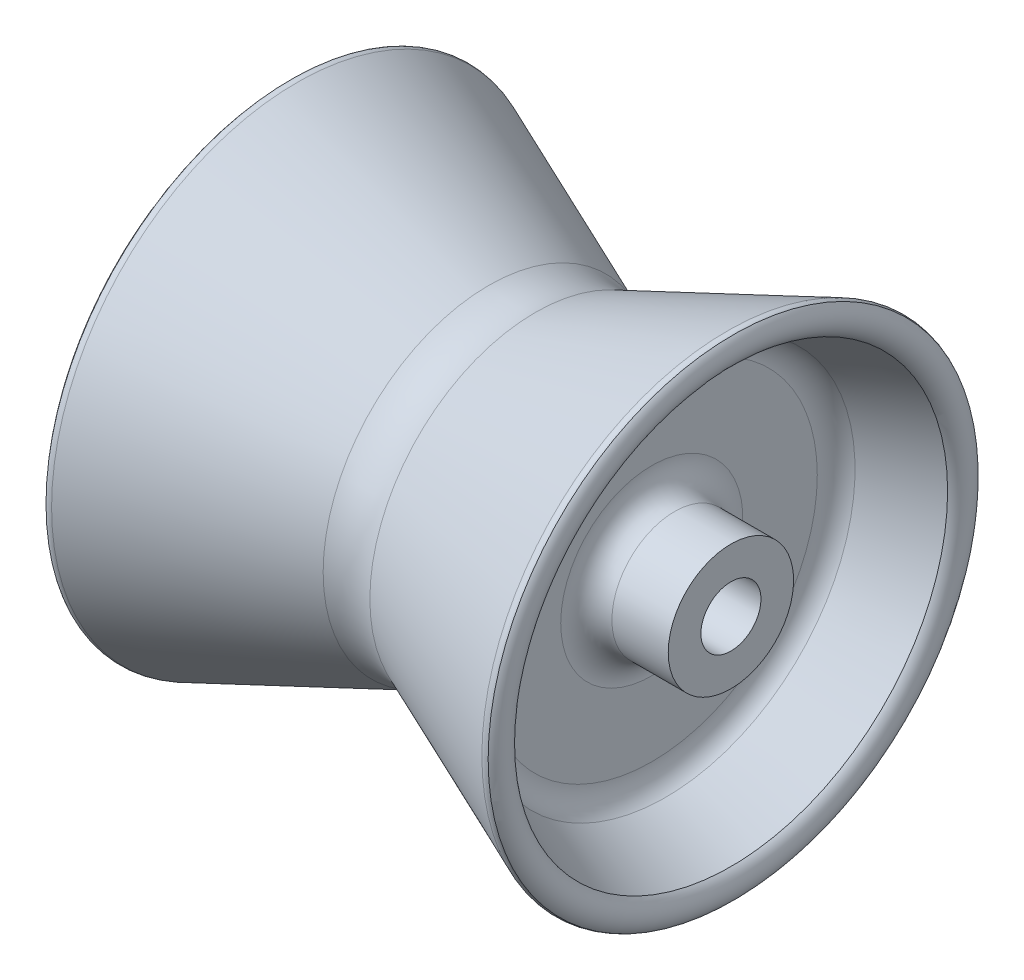
ISO-10303-21;
HEADER;
FILE_DESCRIPTION(('STEP AP214'),'2;1');
FILE_NAME('part.step','',(''),(''),'','','');
FILE_SCHEMA(('AUTOMOTIVE_DESIGN { 1 0 10303 214 1 1 1 1 }'));
ENDSEC;
DATA;
#1=APPLICATION_CONTEXT('core data for automotive mechanical design processes');
#2=APPLICATION_PROTOCOL_DEFINITION('international standard','automotive_design',2000,#1);
#3=PRODUCT_CONTEXT('',#1,'mechanical');
#4=PRODUCT('Part','Part','',(#3));
#5=PRODUCT_RELATED_PRODUCT_CATEGORY('part','',(#4));
#6=PRODUCT_DEFINITION_FORMATION('','',#4);
#7=PRODUCT_DEFINITION_CONTEXT('part definition',#1,'design');
#8=PRODUCT_DEFINITION('design','',#6,#7);
#9=PRODUCT_DEFINITION_SHAPE('','',#8);
#10=(LENGTH_UNIT() NAMED_UNIT(*) SI_UNIT(.MILLI.,.METRE.));
#11=(NAMED_UNIT(*) PLANE_ANGLE_UNIT() SI_UNIT($,.RADIAN.));
#12=(NAMED_UNIT(*) SI_UNIT($,.STERADIAN.) SOLID_ANGLE_UNIT());
#13=UNCERTAINTY_MEASURE_WITH_UNIT(LENGTH_MEASURE(1.E-05),#10,'distance_accuracy_value','');
#14=(GEOMETRIC_REPRESENTATION_CONTEXT(3) GLOBAL_UNCERTAINTY_ASSIGNED_CONTEXT((#13)) GLOBAL_UNIT_ASSIGNED_CONTEXT((#10,
#11,#12)) REPRESENTATION_CONTEXT('',''));
#15=CARTESIAN_POINT('',(0.,0.,0.));
#16=DIRECTION('',(0.,0.,1.));
#17=DIRECTION('',(1.,0.,0.));
#18=AXIS2_PLACEMENT_3D('',#15,#16,#17);
#19=CARTESIAN_POINT('',(166.316369771981,32.5,0.));
#20=DIRECTION('',(-1.,0.,0.));
#21=DIRECTION('',(0.,0.,1.));
#22=AXIS2_PLACEMENT_3D('',#19,#20,#21);
#23=TOROIDAL_SURFACE('',#22,261.095077373778,73.3870314176686);
#24=CARTESIAN_POINT('',(193.537139087232,32.5,0.));
#25=DIRECTION('',(-1.,0.,0.));
#26=DIRECTION('',(0.,0.,1.));
#27=AXIS2_PLACEMENT_3D('',#24,#25,#26);
#28=CIRCLE('',#27,192.943143445358);
#29=CARTESIAN_POINT('',(193.537139087232,32.5,192.943143445358));
#30=VERTEX_POINT('',#29);
#31=EDGE_CURVE('E130',#30,#30,#28,.T.);
#32=ORIENTED_EDGE('',*,*,#31,.T.);
#33=EDGE_LOOP('',(#32));
#34=FACE_BOUND('',#33,.T.);
#35=CARTESIAN_POINT('',(139.095600456727,32.5,0.));
#36=DIRECTION('',(-1.,0.,0.));
#37=DIRECTION('',(0.,0.,1.));
#38=AXIS2_PLACEMENT_3D('',#35,#36,#37);
#39=CIRCLE('',#38,192.943143445359);
#40=CARTESIAN_POINT('',(139.095600456727,32.5,192.943143445359));
#41=VERTEX_POINT('',#40);
#42=EDGE_CURVE('E10',#41,#41,#39,.T.);
#43=ORIENTED_EDGE('',*,*,#42,.F.);
#44=EDGE_LOOP('',(#43));
#45=FACE_BOUND('',#44,.T.);
#46=ADVANCED_FACE('F39',(#34,#45),#23,.F.);
#47=CARTESIAN_POINT('',(139.095600456727,32.5,0.));
#48=DIRECTION('',(-1.,0.,0.));
#49=DIRECTION('',(0.,0.,1.));
#50=AXIS2_PLACEMENT_3D('',#47,#48,#49);
#51=CONICAL_SURFACE('',#50,192.943143445359,0.394231079167529);
#52=CARTESIAN_POINT('',(-84.379337495771,32.5,0.));
#53=DIRECTION('',(-1.,0.,0.));
#54=DIRECTION('',(0.,0.,1.));
#55=AXIS2_PLACEMENT_3D('',#52,#53,#54);
#56=CIRCLE('',#55,285.910851851649);
#57=CARTESIAN_POINT('',(-84.379337495771,32.5,285.910851851649));
#58=VERTEX_POINT('',#57);
#59=EDGE_CURVE('E44',#58,#58,#56,.T.);
#60=ORIENTED_EDGE('',*,*,#59,.F.);
#61=EDGE_LOOP('',(#60));
#62=FACE_BOUND('',#61,.T.);
#63=ORIENTED_EDGE('',*,*,#42,.T.);
#64=EDGE_LOOP('',(#63));
#65=FACE_BOUND('',#64,.T.);
#66=ADVANCED_FACE('F144',(#62,#65),#51,.T.);
#67=CARTESIAN_POINT('',(-87.4080424943852,32.5,0.));
#68=DIRECTION('',(-1.,0.,0.));
#69=DIRECTION('',(0.,0.,1.));
#70=AXIS2_PLACEMENT_3D('',#67,#68,#69);
#71=TOROIDAL_SURFACE('',#70,278.547583622691,7.9618322627528);
#72=CARTESIAN_POINT('',(-91.2932950595249,32.5,0.));
#73=DIRECTION('',(-1.,0.,0.));
#74=DIRECTION('',(0.,0.,1.));
#75=AXIS2_PLACEMENT_3D('',#72,#73,#74);
#76=CIRCLE('',#75,285.497086157786);
#77=CARTESIAN_POINT('',(-91.2932950595249,32.5,285.497086157786));
#78=VERTEX_POINT('',#77);
#79=EDGE_CURVE('E47',#78,#78,#76,.T.);
#80=ORIENTED_EDGE('',*,*,#79,.F.);
#81=EDGE_LOOP('',(#80));
#82=FACE_BOUND('',#81,.T.);
#83=ORIENTED_EDGE('',*,*,#59,.T.);
#84=EDGE_LOOP('',(#83));
#85=FACE_BOUND('',#84,.T.);
#86=ADVANCED_FACE('F149',(#82,#85),#71,.T.);
#87=CARTESIAN_POINT('',(-76.0526601369194,32.5,0.));
#88=DIRECTION('',(-1.,0.,0.));
#89=DIRECTION('',(0.,0.,1.));
#90=AXIS2_PLACEMENT_3D('',#87,#88,#89);
#91=TOROIDAL_SURFACE('',#90,270.101416286388,21.6634162502867);
#92=CARTESIAN_POINT('',(-88.683630228019,32.5,0.));
#93=DIRECTION('',(-1.,0.,0.));
#94=DIRECTION('',(0.,0.,1.));
#95=AXIS2_PLACEMENT_3D('',#92,#93,#94);
#96=CIRCLE('',#95,252.501353837893);
#97=CARTESIAN_POINT('',(-88.683630228019,32.5,252.501353837893));
#98=VERTEX_POINT('',#97);
#99=EDGE_CURVE('E52',#98,#98,#96,.T.);
#100=ORIENTED_EDGE('',*,*,#99,.F.);
#101=EDGE_LOOP('',(#100));
#102=FACE_BOUND('',#101,.T.);
#103=ORIENTED_EDGE('',*,*,#79,.T.);
#104=EDGE_LOOP('',(#103));
#105=FACE_BOUND('',#104,.T.);
#106=ADVANCED_FACE('F152',(#102,#105),#91,.T.);
#107=CARTESIAN_POINT('',(-12.4985969086646,32.5,0.));
#108=DIRECTION('',(-1.,0.,0.));
#109=DIRECTION('',(0.,0.,1.));
#110=AXIS2_PLACEMENT_3D('',#107,#108,#109);
#111=CONICAL_SURFACE('',#110,220.80765239893,0.39423107916753);
#112=ORIENTED_EDGE('',*,*,#99,.T.);
#113=EDGE_LOOP('',(#112));
#114=FACE_BOUND('',#113,.T.);
#115=CARTESIAN_POINT('',(-12.4985969086646,32.5,0.));
#116=DIRECTION('',(-1.,0.,0.));
#117=DIRECTION('',(0.,0.,1.));
#118=AXIS2_PLACEMENT_3D('',#115,#116,#117);
#119=CIRCLE('',#118,220.80765239893);
#120=CARTESIAN_POINT('',(-12.4985969086646,32.5,220.80765239893));
#121=VERTEX_POINT('',#120);
#122=EDGE_CURVE('E59',#121,#121,#119,.T.);
#123=ORIENTED_EDGE('',*,*,#122,.F.);
#124=EDGE_LOOP('',(#123));
#125=FACE_BOUND('',#124,.T.);
#126=ADVANCED_FACE('F159',(#114,#125),#111,.F.);
#127=CARTESIAN_POINT('',(-26.4282593785541,32.5,0.));
#128=DIRECTION('',(-1.,0.,0.));
#129=DIRECTION('',(0.,0.,1.));
#130=AXIS2_PLACEMENT_3D('',#127,#128,#129);
#131=TOROIDAL_SURFACE('',#130,194.237659860826,30.);
#132=ORIENTED_EDGE('',*,*,#122,.T.);
#133=EDGE_LOOP('',(#132));
#134=FACE_BOUND('',#133,.T.);
#135=CARTESIAN_POINT('',(3.54020344965761,32.5,0.));
#136=DIRECTION('',(-1.,0.,0.));
#137=DIRECTION('',(0.,0.,1.));
#138=AXIS2_PLACEMENT_3D('',#135,#136,#137);
#139=CIRCLE('',#138,192.862437800907);
#140=CARTESIAN_POINT('',(3.54020344965761,32.5,192.862437800907));
#141=VERTEX_POINT('',#140);
#142=EDGE_CURVE('E62',#141,#141,#139,.T.);
#143=ORIENTED_EDGE('',*,*,#142,.F.);
#144=EDGE_LOOP('',(#143));
#145=FACE_BOUND('',#144,.T.);
#146=ADVANCED_FACE('F163',(#134,#145),#131,.F.);
#147=CARTESIAN_POINT('',(3.54020344965761,0.,0.));
#148=DIRECTION('',(1.,0.,0.));
#149=DIRECTION('',(0.,0.,-1.));
#150=AXIS2_PLACEMENT_3D('',#147,#148,#149);
#151=PLANE('',#150);
#152=CARTESIAN_POINT('',(3.54020344965761,32.5,0.));
#153=DIRECTION('',(-1.,0.,0.));
#154=DIRECTION('',(0.,0.,1.));
#155=AXIS2_PLACEMENT_3D('',#152,#153,#154);
#156=CIRCLE('',#155,106.114315122698);
#157=CARTESIAN_POINT('',(3.54020344965761,32.5,106.114315122698));
#158=VERTEX_POINT('',#157);
#159=EDGE_CURVE('E61',#158,#158,#156,.T.);
#160=ORIENTED_EDGE('',*,*,#159,.F.);
#161=EDGE_LOOP('',(#160));
#162=FACE_BOUND('',#161,.T.);
#163=ORIENTED_EDGE('',*,*,#142,.T.);
#164=EDGE_LOOP('',(#163));
#165=FACE_BOUND('',#164,.T.);
#166=ADVANCED_FACE('F169',(#162,#165),#151,.F.);
#167=CARTESIAN_POINT('',(-26.2841253791533,32.5,0.));
#168=DIRECTION('',(-1.,0.,0.));
#169=DIRECTION('',(0.,0.,1.));
#170=AXIS2_PLACEMENT_3D('',#167,#168,#169);
#171=TOROIDAL_SURFACE('',#170,102.872493117874,30.);
#172=CARTESIAN_POINT('',(-23.042303374329,32.5,0.));
#173=DIRECTION('',(-1.,0.,0.));
#174=DIRECTION('',(0.,0.,1.));
#175=AXIS2_PLACEMENT_3D('',#172,#173,#174);
#176=CIRCLE('',#175,73.0481642890634);
#177=CARTESIAN_POINT('',(-23.042303374329,32.5,73.0481642890634));
#178=VERTEX_POINT('',#177);
#179=EDGE_CURVE('E69',#178,#178,#176,.T.);
#180=ORIENTED_EDGE('',*,*,#179,.F.);
#181=EDGE_LOOP('',(#180));
#182=FACE_BOUND('',#181,.T.);
#183=ORIENTED_EDGE('',*,*,#159,.T.);
#184=EDGE_LOOP('',(#183));
#185=FACE_BOUND('',#184,.T.);
#186=ADVANCED_FACE('F175',(#182,#185),#171,.F.);
#187=CARTESIAN_POINT('',(-88.6836302280191,32.5,0.));
#188=DIRECTION('',(-1.,0.,0.));
#189=DIRECTION('',(0.,0.,1.));
#190=AXIS2_PLACEMENT_3D('',#187,#188,#189);
#191=CYLINDRICAL_SURFACE('',#190,73.0481642890634);
#192=CARTESIAN_POINT('',(-88.6836302280191,32.5,0.));
#193=DIRECTION('',(-1.,0.,0.));
#194=DIRECTION('',(0.,0.,1.));
#195=AXIS2_PLACEMENT_3D('',#192,#193,#194);
#196=CIRCLE('',#195,73.0481642890634);
#197=CARTESIAN_POINT('',(-88.6836302280191,32.5,73.0481642890634));
#198=VERTEX_POINT('',#197);
#199=EDGE_CURVE('E66',#198,#198,#196,.T.);
#200=ORIENTED_EDGE('',*,*,#199,.F.);
#201=EDGE_LOOP('',(#200));
#202=FACE_BOUND('',#201,.T.);
#203=ORIENTED_EDGE('',*,*,#179,.T.);
#204=EDGE_LOOP('',(#203));
#205=FACE_BOUND('',#204,.T.);
#206=ADVANCED_FACE('F178',(#202,#205),#191,.T.);
#207=CARTESIAN_POINT('',(-88.6836302280191,0.,0.));
#208=DIRECTION('',(1.,0.,0.));
#209=DIRECTION('',(0.,0.,-1.));
#210=AXIS2_PLACEMENT_3D('',#207,#208,#209);
#211=PLANE('',#210);
#212=CARTESIAN_POINT('',(-88.6836302280191,32.5,0.));
#213=DIRECTION('',(-1.,0.,0.));
#214=DIRECTION('',(0.,0.,1.));
#215=AXIS2_PLACEMENT_3D('',#212,#213,#214);
#216=CIRCLE('',#215,34.9895178574439);
#217=CARTESIAN_POINT('',(-88.6836302280191,32.5,34.9895178574439));
#218=VERTEX_POINT('',#217);
#219=EDGE_CURVE('E71',#218,#218,#216,.T.);
#220=ORIENTED_EDGE('',*,*,#219,.F.);
#221=EDGE_LOOP('',(#220));
#222=FACE_BOUND('',#221,.T.);
#223=ORIENTED_EDGE('',*,*,#199,.T.);
#224=EDGE_LOOP('',(#223));
#225=FACE_BOUND('',#224,.T.);
#226=ADVANCED_FACE('F176',(#222,#225),#211,.F.);
#227=CARTESIAN_POINT('',(-88.6836302280191,32.5,0.));
#228=DIRECTION('',(-1.,0.,0.));
#229=DIRECTION('',(0.,0.,1.));
#230=AXIS2_PLACEMENT_3D('',#227,#228,#229);
#231=CYLINDRICAL_SURFACE('',#230,34.9895178574439);
#232=CARTESIAN_POINT('',(44.0541968759562,32.5,0.));
#233=DIRECTION('',(-1.,0.,0.));
#234=DIRECTION('',(0.,0.,1.));
#235=AXIS2_PLACEMENT_3D('',#232,#233,#234);
#236=CIRCLE('',#235,34.9895178574439);
#237=CARTESIAN_POINT('',(44.0541968759562,32.5,34.9895178574439));
#238=VERTEX_POINT('',#237);
#239=EDGE_CURVE('E77',#238,#238,#236,.T.);
#240=ORIENTED_EDGE('',*,*,#239,.F.);
#241=EDGE_LOOP('',(#240));
#242=FACE_BOUND('',#241,.T.);
#243=ORIENTED_EDGE('',*,*,#219,.T.);
#244=EDGE_LOOP('',(#243));
#245=FACE_BOUND('',#244,.T.);
#246=ADVANCED_FACE('F184',(#242,#245),#231,.F.);
#247=CARTESIAN_POINT('',(44.0541968759562,0.,0.));
#248=DIRECTION('',(-1.,0.,0.));
#249=DIRECTION('',(0.,0.,1.));
#250=AXIS2_PLACEMENT_3D('',#247,#248,#249);
#251=PLANE('',#250);
#252=CARTESIAN_POINT('',(44.0541968759562,32.5,0.));
#253=DIRECTION('',(-1.,0.,0.));
#254=DIRECTION('',(0.,0.,1.));
#255=AXIS2_PLACEMENT_3D('',#252,#253,#254);
#256=CIRCLE('',#255,151.408436408375);
#257=CARTESIAN_POINT('',(44.0541968759562,32.5,151.408436408375));
#258=VERTEX_POINT('',#257);
#259=EDGE_CURVE('E76',#258,#258,#256,.T.);
#260=ORIENTED_EDGE('',*,*,#259,.F.);
#261=EDGE_LOOP('',(#260));
#262=FACE_BOUND('',#261,.T.);
#263=ORIENTED_EDGE('',*,*,#239,.T.);
#264=EDGE_LOOP('',(#263));
#265=FACE_BOUND('',#264,.T.);
#266=ADVANCED_FACE('F189',(#262,#265),#251,.F.);
#267=CARTESIAN_POINT('',(74.0384434656632,32.5,0.));
#268=DIRECTION('',(-1.,0.,0.));
#269=DIRECTION('',(0.,0.,1.));
#270=AXIS2_PLACEMENT_3D('',#267,#268,#269);
#271=TOROIDAL_SURFACE('',#270,152.380525111963,30.);
#272=ORIENTED_EDGE('',*,*,#259,.T.);
#273=EDGE_LOOP('',(#272));
#274=FACE_BOUND('',#273,.T.);
#275=CARTESIAN_POINT('',(87.2964364909202,32.5,0.));
#276=DIRECTION('',(-1.,0.,0.));
#277=DIRECTION('',(0.,0.,1.));
#278=AXIS2_PLACEMENT_3D('',#275,#276,#277);
#279=CIRCLE('',#278,179.291965447669);
#280=CARTESIAN_POINT('',(87.2964364909202,32.5,179.291965447669));
#281=VERTEX_POINT('',#280);
#282=EDGE_CURVE('E84',#281,#281,#279,.T.);
#283=ORIENTED_EDGE('',*,*,#282,.F.);
#284=EDGE_LOOP('',(#283));
#285=FACE_BOUND('',#284,.T.);
#286=ADVANCED_FACE('F194',(#274,#285),#271,.F.);
#287=CARTESIAN_POINT('',(126.806403131451,32.5,0.));
#288=DIRECTION('',(-1.,0.,0.));
#289=DIRECTION('',(0.,0.,1.));
#290=AXIS2_PLACEMENT_3D('',#287,#288,#289);
#291=CONICAL_SURFACE('',#290,162.8554419993,0.39423107916753);
#292=ORIENTED_EDGE('',*,*,#282,.T.);
#293=EDGE_LOOP('',(#292));
#294=FACE_BOUND('',#293,.T.);
#295=CARTESIAN_POINT('',(126.806403131451,32.5,0.));
#296=DIRECTION('',(-1.,0.,0.));
#297=DIRECTION('',(0.,0.,1.));
#298=AXIS2_PLACEMENT_3D('',#295,#296,#297);
#299=CIRCLE('',#298,162.8554419993);
#300=CARTESIAN_POINT('',(126.806403131451,32.5,162.8554419993));
#301=VERTEX_POINT('',#300);
#302=EDGE_CURVE('E81',#301,#301,#299,.T.);
#303=ORIENTED_EDGE('',*,*,#302,.F.);
#304=EDGE_LOOP('',(#303));
#305=FACE_BOUND('',#304,.T.);
#306=ADVANCED_FACE('F198',(#294,#305),#291,.F.);
#307=CARTESIAN_POINT('',(166.316369771981,32.5,0.));
#308=DIRECTION('',(-1.,0.,0.));
#309=DIRECTION('',(0.,0.,1.));
#310=AXIS2_PLACEMENT_3D('',#307,#308,#309);
#311=TOROIDAL_SURFACE('',#310,261.095077373778,105.887031417669);
#312=CARTESIAN_POINT('',(205.826336412511,32.5,0.));
#313=DIRECTION('',(-1.,0.,0.));
#314=DIRECTION('',(0.,0.,1.));
#315=AXIS2_PLACEMENT_3D('',#312,#313,#314);
#316=CIRCLE('',#315,162.8554419993);
#317=CARTESIAN_POINT('',(205.826336412511,32.5,162.8554419993));
#318=VERTEX_POINT('',#317);
#319=EDGE_CURVE('E86',#318,#318,#316,.T.);
#320=ORIENTED_EDGE('',*,*,#319,.F.);
#321=EDGE_LOOP('',(#320));
#322=FACE_BOUND('',#321,.T.);
#323=ORIENTED_EDGE('',*,*,#302,.T.);
#324=EDGE_LOOP('',(#323));
#325=FACE_BOUND('',#324,.T.);
#326=ADVANCED_FACE('F199',(#322,#325),#311,.T.);
#327=CARTESIAN_POINT('',(205.826336412511,32.5,0.));
#328=DIRECTION('',(1.,0.,0.));
#329=DIRECTION('',(0.,0.,-1.));
#330=AXIS2_PLACEMENT_3D('',#327,#328,#329);
#331=CONICAL_SURFACE('',#330,162.8554419993,0.39423107916753);
#332=CARTESIAN_POINT('',(245.336303053042,32.5,0.));
#333=DIRECTION('',(-1.,0.,0.));
#334=DIRECTION('',(0.,0.,1.));
#335=AXIS2_PLACEMENT_3D('',#332,#333,#334);
#336=CIRCLE('',#335,179.291965447669);
#337=CARTESIAN_POINT('',(245.336303053042,32.5,179.291965447669));
#338=VERTEX_POINT('',#337);
#339=EDGE_CURVE('E93',#338,#338,#336,.T.);
#340=ORIENTED_EDGE('',*,*,#339,.F.);
#341=EDGE_LOOP('',(#340));
#342=FACE_BOUND('',#341,.T.);
#343=ORIENTED_EDGE('',*,*,#319,.T.);
#344=EDGE_LOOP('',(#343));
#345=FACE_BOUND('',#344,.T.);
#346=ADVANCED_FACE('F204',(#342,#345),#331,.F.);
#347=CARTESIAN_POINT('',(258.594296078299,32.5,0.));
#348=DIRECTION('',(-1.,0.,0.));
#349=DIRECTION('',(0.,0.,1.));
#350=AXIS2_PLACEMENT_3D('',#347,#348,#349);
#351=TOROIDAL_SURFACE('',#350,152.380525111963,30.);
#352=CARTESIAN_POINT('',(288.578542668006,32.5,0.));
#353=DIRECTION('',(-1.,0.,0.));
#354=DIRECTION('',(0.,0.,1.));
#355=AXIS2_PLACEMENT_3D('',#352,#353,#354);
#356=CIRCLE('',#355,151.408436408375);
#357=CARTESIAN_POINT('',(288.578542668006,32.5,151.408436408375));
#358=VERTEX_POINT('',#357);
#359=EDGE_CURVE('E94',#358,#358,#356,.T.);
#360=ORIENTED_EDGE('',*,*,#359,.F.);
#361=EDGE_LOOP('',(#360));
#362=FACE_BOUND('',#361,.T.);
#363=ORIENTED_EDGE('',*,*,#339,.T.);
#364=EDGE_LOOP('',(#363));
#365=FACE_BOUND('',#364,.T.);
#366=ADVANCED_FACE('F208',(#362,#365),#351,.F.);
#367=CARTESIAN_POINT('',(288.578542668006,0.,0.));
#368=DIRECTION('',(-1.,0.,0.));
#369=DIRECTION('',(0.,0.,1.));
#370=AXIS2_PLACEMENT_3D('',#367,#368,#369);
#371=PLANE('',#370);
#372=ORIENTED_EDGE('',*,*,#359,.T.);
#373=EDGE_LOOP('',(#372));
#374=FACE_BOUND('',#373,.T.);
#375=CARTESIAN_POINT('',(288.578542668006,32.5,0.));
#376=DIRECTION('',(-1.,0.,0.));
#377=DIRECTION('',(0.,0.,1.));
#378=AXIS2_PLACEMENT_3D('',#375,#376,#377);
#379=CIRCLE('',#378,34.989517857444);
#380=CARTESIAN_POINT('',(288.578542668006,32.5,34.989517857444));
#381=VERTEX_POINT('',#380);
#382=EDGE_CURVE('E100',#381,#381,#379,.T.);
#383=ORIENTED_EDGE('',*,*,#382,.F.);
#384=EDGE_LOOP('',(#383));
#385=FACE_BOUND('',#384,.T.);
#386=ADVANCED_FACE('F215',(#374,#385),#371,.T.);
#387=CARTESIAN_POINT('',(-88.6836302280191,32.5,0.));
#388=DIRECTION('',(-1.,0.,0.));
#389=DIRECTION('',(0.,0.,1.));
#390=AXIS2_PLACEMENT_3D('',#387,#388,#389);
#391=CYLINDRICAL_SURFACE('',#390,34.989517857444);
#392=ORIENTED_EDGE('',*,*,#382,.T.);
#393=EDGE_LOOP('',(#392));
#394=FACE_BOUND('',#393,.T.);
#395=CARTESIAN_POINT('',(421.316369771981,32.5,0.));
#396=DIRECTION('',(-1.,0.,0.));
#397=DIRECTION('',(0.,0.,1.));
#398=AXIS2_PLACEMENT_3D('',#395,#396,#397);
#399=CIRCLE('',#398,34.989517857444);
#400=CARTESIAN_POINT('',(421.316369771981,32.5,34.989517857444));
#401=VERTEX_POINT('',#400);
#402=EDGE_CURVE('E99',#401,#401,#399,.T.);
#403=ORIENTED_EDGE('',*,*,#402,.F.);
#404=EDGE_LOOP('',(#403));
#405=FACE_BOUND('',#404,.T.);
#406=ADVANCED_FACE('F216',(#394,#405),#391,.F.);
#407=CARTESIAN_POINT('',(421.316369771981,0.,0.));
#408=DIRECTION('',(1.,0.,0.));
#409=DIRECTION('',(0.,0.,-1.));
#410=AXIS2_PLACEMENT_3D('',#407,#408,#409);
#411=PLANE('',#410);
#412=ORIENTED_EDGE('',*,*,#402,.T.);
#413=EDGE_LOOP('',(#412));
#414=FACE_BOUND('',#413,.T.);
#415=CARTESIAN_POINT('',(421.316369771981,32.5,0.));
#416=DIRECTION('',(-1.,0.,0.));
#417=DIRECTION('',(0.,0.,1.));
#418=AXIS2_PLACEMENT_3D('',#415,#416,#417);
#419=CIRCLE('',#418,73.0481642890635);
#420=CARTESIAN_POINT('',(421.316369771981,32.5,73.0481642890635));
#421=VERTEX_POINT('',#420);
#422=EDGE_CURVE('E103',#421,#421,#419,.T.);
#423=ORIENTED_EDGE('',*,*,#422,.F.);
#424=EDGE_LOOP('',(#423));
#425=FACE_BOUND('',#424,.T.);
#426=ADVANCED_FACE('F219',(#414,#425),#411,.T.);
#427=CARTESIAN_POINT('',(-88.6836302280191,32.5,0.));
#428=DIRECTION('',(-1.,0.,0.));
#429=DIRECTION('',(0.,0.,1.));
#430=AXIS2_PLACEMENT_3D('',#427,#428,#429);
#431=CYLINDRICAL_SURFACE('',#430,73.0481642890635);
#432=ORIENTED_EDGE('',*,*,#422,.T.);
#433=EDGE_LOOP('',(#432));
#434=FACE_BOUND('',#433,.T.);
#435=CARTESIAN_POINT('',(355.675042918291,32.5,0.));
#436=DIRECTION('',(-1.,0.,0.));
#437=DIRECTION('',(0.,0.,1.));
#438=AXIS2_PLACEMENT_3D('',#435,#436,#437);
#439=CIRCLE('',#438,73.0481642890635);
#440=CARTESIAN_POINT('',(355.675042918291,32.5,73.0481642890635));
#441=VERTEX_POINT('',#440);
#442=EDGE_CURVE('E106',#441,#441,#439,.T.);
#443=ORIENTED_EDGE('',*,*,#442,.F.);
#444=EDGE_LOOP('',(#443));
#445=FACE_BOUND('',#444,.T.);
#446=ADVANCED_FACE('F221',(#434,#445),#431,.T.);
#447=CARTESIAN_POINT('',(358.916864923115,32.5,0.));
#448=DIRECTION('',(-1.,0.,0.));
#449=DIRECTION('',(0.,0.,1.));
#450=AXIS2_PLACEMENT_3D('',#447,#448,#449);
#451=TOROIDAL_SURFACE('',#450,102.872493117874,30.);
#452=ORIENTED_EDGE('',*,*,#442,.T.);
#453=EDGE_LOOP('',(#452));
#454=FACE_BOUND('',#453,.T.);
#455=CARTESIAN_POINT('',(329.092536094304,32.5,0.));
#456=DIRECTION('',(-1.,0.,0.));
#457=DIRECTION('',(0.,0.,1.));
#458=AXIS2_PLACEMENT_3D('',#455,#456,#457);
#459=CIRCLE('',#458,106.114315122698);
#460=CARTESIAN_POINT('',(329.092536094304,32.5,106.114315122698));
#461=VERTEX_POINT('',#460);
#462=EDGE_CURVE('E108',#461,#461,#459,.T.);
#463=ORIENTED_EDGE('',*,*,#462,.F.);
#464=EDGE_LOOP('',(#463));
#465=FACE_BOUND('',#464,.T.);
#466=ADVANCED_FACE('F229',(#454,#465),#451,.F.);
#467=CARTESIAN_POINT('',(329.092536094304,0.,0.));
#468=DIRECTION('',(1.,0.,0.));
#469=DIRECTION('',(0.,0.,-1.));
#470=AXIS2_PLACEMENT_3D('',#467,#468,#469);
#471=PLANE('',#470);
#472=ORIENTED_EDGE('',*,*,#462,.T.);
#473=EDGE_LOOP('',(#472));
#474=FACE_BOUND('',#473,.T.);
#475=CARTESIAN_POINT('',(329.092536094304,32.5,0.));
#476=DIRECTION('',(-1.,0.,0.));
#477=DIRECTION('',(0.,0.,1.));
#478=AXIS2_PLACEMENT_3D('',#475,#476,#477);
#479=CIRCLE('',#478,192.862437800906);
#480=CARTESIAN_POINT('',(329.092536094304,32.5,192.862437800906));
#481=VERTEX_POINT('',#480);
#482=EDGE_CURVE('E115',#481,#481,#479,.T.);
#483=ORIENTED_EDGE('',*,*,#482,.F.);
#484=EDGE_LOOP('',(#483));
#485=FACE_BOUND('',#484,.T.);
#486=ADVANCED_FACE('F234',(#474,#485),#471,.T.);
#487=CARTESIAN_POINT('',(359.060998922516,32.5,0.));
#488=DIRECTION('',(-1.,0.,0.));
#489=DIRECTION('',(0.,0.,1.));
#490=AXIS2_PLACEMENT_3D('',#487,#488,#489);
#491=TOROIDAL_SURFACE('',#490,194.237659860826,30.);
#492=CARTESIAN_POINT('',(345.131336452626,32.5,0.));
#493=DIRECTION('',(-1.,0.,0.));
#494=DIRECTION('',(0.,0.,1.));
#495=AXIS2_PLACEMENT_3D('',#492,#493,#494);
#496=CIRCLE('',#495,220.807652398931);
#497=CARTESIAN_POINT('',(345.131336452626,32.5,220.807652398931));
#498=VERTEX_POINT('',#497);
#499=EDGE_CURVE('E113',#498,#498,#496,.T.);
#500=ORIENTED_EDGE('',*,*,#499,.F.);
#501=EDGE_LOOP('',(#500));
#502=FACE_BOUND('',#501,.T.);
#503=ORIENTED_EDGE('',*,*,#482,.T.);
#504=EDGE_LOOP('',(#503));
#505=FACE_BOUND('',#504,.T.);
#506=ADVANCED_FACE('F237',(#502,#505),#491,.F.);
#507=CARTESIAN_POINT('',(345.131336452626,32.5,0.));
#508=DIRECTION('',(1.,0.,0.));
#509=DIRECTION('',(0.,0.,-1.));
#510=AXIS2_PLACEMENT_3D('',#507,#508,#509);
#511=CONICAL_SURFACE('',#510,220.807652398931,0.39423107916753);
#512=CARTESIAN_POINT('',(421.316369771981,32.5,0.));
#513=DIRECTION('',(-1.,0.,0.));
#514=DIRECTION('',(0.,0.,1.));
#515=AXIS2_PLACEMENT_3D('',#512,#513,#514);
#516=CIRCLE('',#515,252.501353837894);
#517=CARTESIAN_POINT('',(421.316369771981,32.5,252.501353837894));
#518=VERTEX_POINT('',#517);
#519=EDGE_CURVE('E119',#518,#518,#516,.T.);
#520=ORIENTED_EDGE('',*,*,#519,.F.);
#521=EDGE_LOOP('',(#520));
#522=FACE_BOUND('',#521,.T.);
#523=ORIENTED_EDGE('',*,*,#499,.T.);
#524=EDGE_LOOP('',(#523));
#525=FACE_BOUND('',#524,.T.);
#526=ADVANCED_FACE('F238',(#522,#525),#511,.F.);
#527=CARTESIAN_POINT('',(408.685399680881,32.5,0.));
#528=DIRECTION('',(-1.,0.,0.));
#529=DIRECTION('',(0.,0.,1.));
#530=AXIS2_PLACEMENT_3D('',#527,#528,#529);
#531=TOROIDAL_SURFACE('',#530,270.101416286389,21.6634162502867);
#532=ORIENTED_EDGE('',*,*,#519,.T.);
#533=EDGE_LOOP('',(#532));
#534=FACE_BOUND('',#533,.T.);
#535=CARTESIAN_POINT('',(423.926034603487,32.5,0.));
#536=DIRECTION('',(-1.,0.,0.));
#537=DIRECTION('',(0.,0.,1.));
#538=AXIS2_PLACEMENT_3D('',#535,#536,#537);
#539=CIRCLE('',#538,285.497086157786);
#540=CARTESIAN_POINT('',(423.926034603487,32.5,285.497086157786));
#541=VERTEX_POINT('',#540);
#542=EDGE_CURVE('E123',#541,#541,#539,.T.);
#543=ORIENTED_EDGE('',*,*,#542,.F.);
#544=EDGE_LOOP('',(#543));
#545=FACE_BOUND('',#544,.T.);
#546=ADVANCED_FACE('F143',(#534,#545),#531,.T.);
#547=CARTESIAN_POINT('',(420.040782038347,32.5,0.));
#548=DIRECTION('',(-1.,0.,0.));
#549=DIRECTION('',(0.,0.,1.));
#550=AXIS2_PLACEMENT_3D('',#547,#548,#549);
#551=TOROIDAL_SURFACE('',#550,278.547583622691,7.9618322627528);
#552=ORIENTED_EDGE('',*,*,#542,.T.);
#553=EDGE_LOOP('',(#552));
#554=FACE_BOUND('',#553,.T.);
#555=CARTESIAN_POINT('',(417.012077039733,32.5,0.));
#556=DIRECTION('',(-1.,0.,0.));
#557=DIRECTION('',(0.,0.,1.));
#558=AXIS2_PLACEMENT_3D('',#555,#556,#557);
#559=CIRCLE('',#558,285.910851851649);
#560=CARTESIAN_POINT('',(417.012077039733,32.5,285.910851851649));
#561=VERTEX_POINT('',#560);
#562=EDGE_CURVE('E125',#561,#561,#559,.T.);
#563=ORIENTED_EDGE('',*,*,#562,.F.);
#564=EDGE_LOOP('',(#563));
#565=FACE_BOUND('',#564,.T.);
#566=ADVANCED_FACE('F133',(#554,#565),#551,.T.);
#567=CARTESIAN_POINT('',(193.537139087232,32.5,0.));
#568=DIRECTION('',(1.,0.,0.));
#569=DIRECTION('',(0.,0.,-1.));
#570=AXIS2_PLACEMENT_3D('',#567,#568,#569);
#571=CONICAL_SURFACE('',#570,192.943143445358,0.39423107916753);
#572=ORIENTED_EDGE('',*,*,#562,.T.);
#573=EDGE_LOOP('',(#572));
#574=FACE_BOUND('',#573,.T.);
#575=ORIENTED_EDGE('',*,*,#31,.F.);
#576=EDGE_LOOP('',(#575));
#577=FACE_BOUND('',#576,.T.);
#578=ADVANCED_FACE('F134',(#574,#577),#571,.T.);
#579=CLOSED_SHELL('',(#46,#66,#86,#106,#126,#146,#166,#186,#206,#226,#246,#266,#286,#306,#326,
#346,#366,#386,#406,#426,#446,#466,#486,#506,#526,#546,#566,#578));
#580=MANIFOLD_SOLID_BREP('B2',#579);
#581=ADVANCED_BREP_SHAPE_REPRESENTATION('',(#18,#580),#14);
#582=SHAPE_DEFINITION_REPRESENTATION(#9,#581);
ENDSEC;
END-ISO-10303-21;
